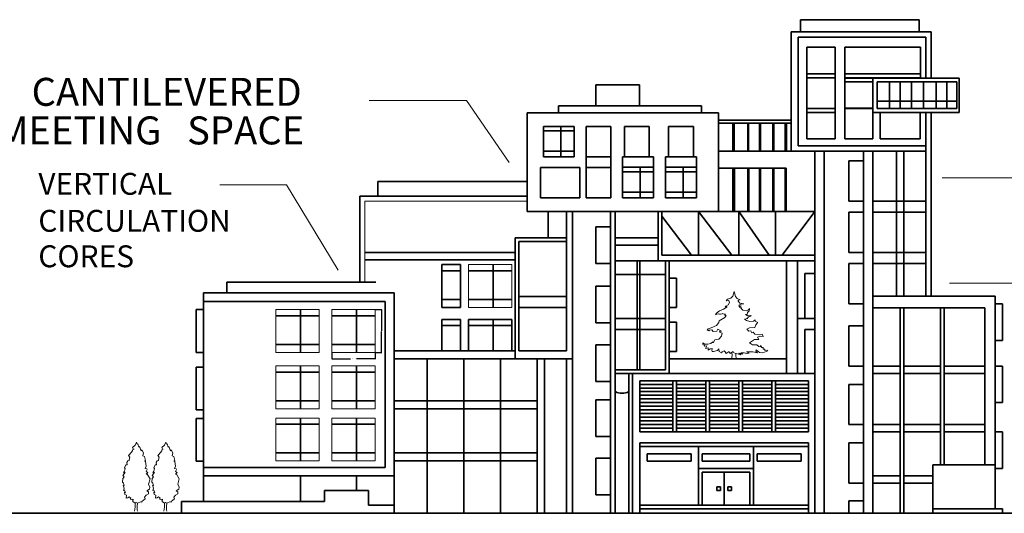
# Model space of a CAD drawing. Units: inches. Extents: x -1080 to 1950, y -1929 to 857.
# Tile 15 of 16: x 769 to 1335, y 9 to 293. Entities that reach past the tile are written whole.
import ezdxf

# ---------------------------------------------------------------- set-up
doc = ezdxf.new("R2010")
doc.units = ezdxf.units.IN
doc.header["$MEASUREMENT"] = 0
for name, color, linetype, lineweight in [('A-ANNO-DIMS', 2, 'Continuous', 18), ('A-ANNO-SYMB', 2, 'Continuous', 18), ('A-ANNO-TEXT', 7, 'Continuous', 25), ('A-ELEV', 7, 'Continuous', 35), ('A-GLAZ', 4, 'Continuous', 18), ('L-PLNT', 82, 'Continuous', 13)]:
    doc.layers.add(name, color=color, linetype=linetype, lineweight=lineweight)
doc.styles.get("Standard").update_dxf_attribs({"font": 'arial.ttf'})
doc.dimstyles.get("Standard").update_dxf_attribs({"dimtxt": 0.18, "dimasz": 0.18, "dimexe": 0.18, "dimexo": 0.0625, "dimgap": 0.09, "dimtad": 0, "dimtih": 1, "dimtoh": 1, "dimdec": 4, "dimzin": 0, "dimdsep": 46, "dimtxsty": 'Standard', "dimcen": 0.09, "dimadec": 0, "dimazin": 0, "dimtfac": 1, "dimtdec": 4, "dimtofl": 0, "dimtmove": 0, "dimatfit": 3, "dimfxl": 1, "dimtolj": 1, "dimtzin": 0, "dimarcsym": 0})

# ---------------------------------------------------------------- blocks, each defined once
blk = doc.blocks.new('*U11')
blk.add_lwpolyline([(-69.9516, 4869.1546), (-172.212, 4644.4154), (-347.5228, 4494.6062), (-303.6824, 4400.9564), (-245.2624, 4382.2366), (-362.1278, 4326.0518), (-347.5228, 4251.1472), (-552.0182, 4007.6882), (-639.6736, 3932.7836), (-537.4132, 3820.414), (-552.0182, 3745.5094), (-581.2536, 3576.955), (-668.8836, 3558.2098), (-741.934, 3427.1204), (-727.329, 3277.3112), (-829.5894, 3258.5914), (-917.2194, 3052.572), (-873.4044, 3015.1324), (-902.6144, 2827.8582), (-990.2698, 2696.7434), (-873.4044, 2734.2084), (-1034.0848, 2509.4692), (-946.4294, 2434.5646), (-1034.0848, 2303.4752), (-1048.6898, 2041.2964), (-975.6648, 1985.1116), (-931.8244, 1797.8374), (-1004.8748, 1816.5572), (-946.4294, 1629.283), (-975.6648, 1460.7286), (-917.2194, 1479.4738), (-844.1944, 1329.6392), (-902.6144, 1348.3844), (-888.0094, 1179.83), (-771.144, 1142.365), (-800.354, 917.6512), (-668.8836, 936.371), (-595.8586, 1011.2756), (-464.3882, 917.6512), (-508.2032, 842.7212), (-376.7328, 805.2816), (-303.6824, 842.7212), (-318.2874, 692.912), (-157.607, 580.5424), (-99.187, 618.0074), (3.0734, 580.5424), (207.5942, 674.1922), (295.2496, 636.7272), (309.8546, 692.912), (543.56, 880.1862), (499.745, 992.5558), (602.0054, 1142.365), (762.6858, 1217.2696), (777.2908, 1367.1042), (645.8204, 1442.0088), (835.7362, 1554.3784), (864.9462, 1704.1876), (777.2908, 1910.207), (879.5512, 2284.7554), (675.0304, 2621.8388), (602.0054, 2621.8388), (718.8708, 2734.2084), (602.0054, 2809.113), (675.0304, 2940.2024), (645.8204, 2996.3872), (528.955, 3015.1324), (616.6104, 3164.9416), (572.7954, 3502.0504), (485.14, 3539.49), (572.7954, 3576.955), (499.745, 3857.8536), (368.2746, 3895.3186), (412.0896, 4120.0578), (309.8546, 4326.0518), (266.0142, 4251.1472), (149.1488, 4550.791), (105.3338, 4513.326), (17.6784, 4756.785), (-11.5316, 4719.32)], close=True)
for points in [[(-173.0502, 601.1926), (-173.0502, 296.3926), (-219.1258, 0)], [(9.8298, 601.1926), (-14.6304, 337.0834), (-14.6304, 93.6244), (0, 0)]]:
    blk.add_lwpolyline(points)
blk = doc.blocks.new('*U7')
blk.add_lwpolyline([(-69.9516, 4869.1546), (-172.212, 4644.4154), (-347.5228, 4494.6062), (-303.6824, 4400.9564), (-245.2624, 4382.2366), (-362.1278, 4326.0518), (-347.5228, 4251.1472), (-552.0182, 4007.6882), (-639.6736, 3932.7836), (-537.4132, 3820.414), (-552.0182, 3745.5094), (-581.2536, 3576.955), (-668.8836, 3558.2098), (-741.934, 3427.1204), (-727.329, 3277.3112), (-829.5894, 3258.5914), (-917.2194, 3052.572), (-873.4044, 3015.1324), (-902.6144, 2827.8582), (-990.2698, 2696.7434), (-873.4044, 2734.2084), (-1034.0848, 2509.4692), (-946.4294, 2434.5646), (-1034.0848, 2303.4752), (-1048.6898, 2041.2964), (-975.6648, 1985.1116), (-931.8244, 1797.8374), (-1004.8748, 1816.5572), (-946.4294, 1629.283), (-975.6648, 1460.7286), (-917.2194, 1479.4738), (-844.1944, 1329.6392), (-902.6144, 1348.3844), (-888.0094, 1179.83), (-771.144, 1142.365), (-800.354, 917.6512), (-668.8836, 936.371), (-595.8586, 1011.2756), (-464.3882, 917.6512), (-508.2032, 842.7212), (-376.7328, 805.2816), (-303.6824, 842.7212), (-318.2874, 692.912), (-157.607, 580.5424), (-99.187, 618.0074), (3.0734, 580.5424), (207.5942, 674.1922), (295.2496, 636.7272), (309.8546, 692.912), (543.56, 880.1862), (499.745, 992.5558), (602.0054, 1142.365), (762.6858, 1217.2696), (777.2908, 1367.1042), (645.8204, 1442.0088), (835.7362, 1554.3784), (864.9462, 1704.1876), (777.2908, 1910.207), (879.5512, 2284.7554), (675.0304, 2621.8388), (602.0054, 2621.8388), (718.8708, 2734.2084), (602.0054, 2809.113), (675.0304, 2940.2024), (645.8204, 2996.3872), (528.955, 3015.1324), (616.6104, 3164.9416), (572.7954, 3502.0504), (485.14, 3539.49), (572.7954, 3576.955), (499.745, 3857.8536), (368.2746, 3895.3186), (412.0896, 4120.0578), (309.8546, 4326.0518), (266.0142, 4251.1472), (149.1488, 4550.791), (105.3338, 4513.326), (17.6784, 4756.785), (-11.5316, 4719.32)], close=True)
for points in [[(-173.0502, 601.1926), (-173.0502, 296.3926), (-219.1258, 0)], [(9.8298, 601.1926), (-14.6304, 337.0834), (-14.6304, 93.6244), (0, 0)]]:
    blk.add_lwpolyline(points)
blk = doc.blocks.new('*U10')
for p, q in [((-247.65, 0), (-209.8802, 192.9892)), ((-209.8802, 192.9892), (-222.1738, 358.267)), ((-19.5834, 242.824), (-17.526, 300.5582)), ((0, 0), (-19.5834, 242.824))]:
    blk.add_line(p, q)
for points in [[(-99.06, 3615.69), (-167.5384, 3353.7398), (-274.3454, 3262.4522), (-452.374, 3201.5938), (-523.5956, 3110.2808), (-452.374, 3140.71), (-381.1778, 3125.4954), (-345.567, 3018.9932), (-428.6504, 2897.251), (-547.3446, 2821.178), (-582.9554, 2790.7488), (-487.9848, 2805.9634), (-499.872, 2775.5342), (-666.0388, 2669.0066), (-879.6782, 2577.719), (-1045.845, 2456.0022), (-1105.1794, 2364.6892), (-1045.845, 2395.1184), (-939.0126, 2425.5476), (-879.6782, 2395.1184), (-832.2056, 2395.1184), (-749.1222, 2425.5476)], [(-95.4786, 3606.038), (-27.2796, 3343.7322), (61.8998, 3229.3814), (224.536, 3162.1222), (166.8272, 3162.1222), (103.886, 3128.4926), (109.1184, 3094.8884), (198.2978, 2993.9996), (408.1526, 2946.908), (266.4968, 2926.7404), (140.589, 2879.6488), (177.3174, 2866.2122), (151.0792, 2819.1206), (261.2644, 2846.0192), (172.085, 2778.7854), (297.9928, 2745.1558), (250.7742, 2724.9628), (350.4438, 2603.9064), (555.0408, 2570.2768), (659.9682, 2637.536), (712.4192, 2704.7952), (707.1868, 2671.1656), (696.6966, 2577.0078), (612.7496, 2482.85), (586.5114, 2375.2302), (497.332, 2375.2302), (597.027, 2328.164), (717.677, 2307.9964), (812.1142, 2334.895), (738.6574, 2281.0724), (623.2398, 2254.1738), (680.9486, 2240.7372), (570.7888, 2186.9146), (633.73, 2173.478), (439.6232, 2139.8484), (555.0408, 2052.4216), (738.6574, 2012.061), (932.7642, 2032.2286), (1011.4534, 2092.7568), (1016.7112, 2032.2286), (1153.1092, 1944.8018)], [(-742.95, 2426.97), (-642.2898, 2395.1184), (-559.2064, 2395.1184), (-606.679, 2319.0454), (-523.5956, 2319.0454), (-594.8172, 2212.5432), (-903.4018, 2045.1572), (-915.289, 1953.8696), (-1045.845, 1786.4836), (-1330.6806, 1664.7668), (-1496.8474, 1619.0976), (-1544.32, 1558.2392), (-1449.3748, 1512.5954), (-1425.6512, 1543.0246), (-1295.0698, 1558.2392), (-1223.8736, 1466.9516), (-1033.9578, 1497.3808), (-974.6234, 1588.6684), (-772.8458, 1482.1662), (-855.9292, 1482.1662), (-891.54, 1436.5224), (-749.1222, 1375.6386), (-784.7076, 1223.4926), (-915.289, 1056.1066), (-1128.9284, 1025.6774), (-1223.8736, 858.2914), (-1247.5972, 919.1752), (-1342.5678, 827.8622), (-1508.7346, 797.433), (-1663.0142, 797.433), (-1781.7084, 873.506), (-1769.8466, 782.2184), (-1698.625, 736.5746), (-1674.9014, 690.9308), (-1556.2072, 706.1454), (-1639.2906, 569.1886), (-1484.9856, 599.6178), (-1484.9856, 477.901), (-1378.1532, 538.7594), (-1259.4844, 553.974), (-1295.0698, 477.901), (-1283.208, 401.828), (-1200.1246, 401.828), (-998.3724, 462.6864), (-927.1508, 538.7594), (-903.4018, 401.828), (-772.8458, 340.9442), (-749.1222, 386.6134), (-642.2898, 432.2572), (-582.9554, 386.6134), (-535.4574, 295.3004), (-369.2906, 401.828), (-333.7052, 295.3004), (-155.6512, 401.828), (-120.0404, 325.7296), (259.7404, 234.442), (141.0716, 310.515), (342.8238, 264.8712), (259.7404, 325.7296), (425.9072, 340.9442), (568.3504, 295.3004), (698.9064, 310.515), (556.4886, 386.6134), (888.8222, 386.6134), (1138.0724, 325.7296), (1054.989, 417.0426), (1078.7126, 493.1156), (1244.8794, 356.1842), (1434.7698, 340.9442), (1695.9072, 432.2572), (1636.5474, 477.901), (1529.7404, 462.6864), (1529.7404, 523.5448), (1446.657, 523.5448), (1446.657, 614.8324), (1375.4354, 614.8324), (1304.2392, 721.36), (1280.4902, 660.5016), (1209.2686, 675.7162), (1114.3234, 767.0038), (983.7674, 767.0038), (876.935, 767.0038), (710.7682, 858.2914), (983.7674, 1040.892), (1209.2686, 1040.892), (1149.9342, 1162.6342), (1327.9628, 1223.4926), (1446.657, 1208.278), (1399.1844, 1329.9948), (1233.0176, 1299.5656), (995.6292, 1329.9948), (912.5458, 1436.5224), (841.3242, 1406.0678), (793.8516, 1512.5954), (687.0446, 1482.1662), (568.3504, 1588.6684), (722.6554, 1664.7668), (995.6292, 1695.196), (1054.989, 1832.1274), (1149.9342, 1938.655)]]:
    blk.add_lwpolyline(points)
blk = doc.blocks.new('WIN-SQUARE')
for p, q in [((0, 24.67), (0, 0)), ((24.91, 24.67), (0, 24.67)), ((24.91, 0), (24.91, 24.67)), ((0, 0), (24.91, 0))]:
    blk.add_line(p, q)
blk = doc.blocks.new('*D69')
at = {"layer": 'A-ANNO-DIMS', "color": 0, "lineweight": -2, "transparency": 16777216}
for p, q in [((948.5, 101.5), (948.5, 97.65)), ((948.68, 97.83), (959.27, 97.83)), ((973.22, 97.83), (962.63, 97.83)), ((973.4, 101.5), (973.4, 97.65))]:
    blk.add_line(p, q, dxfattribs=at)
at = {"layer": 'A-ANNO-DIMS', "color": 0, "transparency": 16777216}
for points in [[(948.68, 97.86), (948.68, 97.8), (948.5, 97.83)], [(973.22, 97.86), (973.22, 97.8), (973.4, 97.83)]]:
    blk.add_solid(points, dxfattribs=at)
at = {"layer": 'Defpoints', "color": 0, "transparency": 16777216}
for p in [(948.5, 101.56), (973.4, 101.56), (973.4, 97.83)]:
    blk.add_point(p, dxfattribs=at)
at = {"layer": 'A-ANNO-DIMS', "color": 0, "transparency": 16777216, "insert": (960.95, 97.83), "char_height": 0.18, "attachment_point": 5}
blk.add_mtext('\\A1;SQUARE WINDOW 25 TYP.', dxfattribs=at)
blk = doc.blocks.new('*D70')
at = {"layer": 'A-ANNO-DIMS', "color": 0, "lineweight": -2, "transparency": 16777216}
for p, q in [((973.47, 126.24), (977.32, 126.24)), ((977.14, 126.06), (977.14, 114.08)), ((977.14, 101.74), (977.14, 113.72)), ((973.47, 101.56), (977.32, 101.56))]:
    blk.add_line(p, q, dxfattribs=at)
at = {"layer": 'A-ANNO-DIMS', "color": 0, "transparency": 16777216}
for points in [[(977.11, 126.06), (977.17, 126.06), (977.14, 126.24)], [(977.11, 101.74), (977.17, 101.74), (977.14, 101.56)]]:
    blk.add_solid(points, dxfattribs=at)
at = {"layer": 'Defpoints', "color": 0, "transparency": 16777216}
for p in [(973.4, 126.24), (977.14, 126.24), (973.4, 101.56)]:
    blk.add_point(p, dxfattribs=at)
at = {"layer": 'A-ANNO-DIMS', "color": 0, "transparency": 16777216, "insert": (977.14, 113.9), "char_height": 0.18, "attachment_point": 5}
blk.add_mtext('\\A1;25 TYP.', dxfattribs=at)

msp = doc.modelspace()

# ---------------------------------------------------------------- linework, layer by layer
at = {"layer": 'A-ANNO-SYMB'}
for p, q in [((1026.06, 246.75), (969.93, 246.75)), ((1050.5, 211.03), (1026.06, 246.75)), ((1299.6, 202.14), (1345.49, 202.14)), ((922.34, 198.18), (884.13, 198.18)), ((952.21, 148.89), (922.34, 198.18)), ((967.5, 142.06), (967.5, 188.65)), ((967.5, 188.65), (1060.92, 188.65)), ((1303.79, 141.55), (1392.21, 141.55))]:
    msp.add_line(p, q, dxfattribs=at)
at = {"layer": 'A-ELEV'}
for p, q in [((1218.17, 286.27), (1218.17, 293.2)), ((1218.17, 293.2), (1286.45, 293.2)), ((1286.45, 293.2), (1286.45, 286.27)), ((1212.83, 217.57), (1212.83, 286.27)), ((1212.83, 286.27), (1293.18, 286.27)), ((1216.68, 283.21), (1290.25, 283.21)), ((1216.68, 220.51), (1216.68, 283.21)), ((1290.25, 283.21), (1290.25, 259.53)), ((1293.18, 286.27), (1293.18, 259.53)), ((1221.83, 277.33), (1238.06, 277.33)), ((1221.83, 224.58), (1221.83, 277.33)), ((1238.06, 277.33), (1238.06, 224.58)), ((1243.54, 277.33), (1243.54, 261.97)), ((1287.05, 277.33), (1243.54, 277.33)), ((1287.05, 261.97), (1287.05, 277.33)), ((1238.06, 261.97), (1221.83, 261.97)), ((1243.54, 261.97), (1287.05, 261.97)), ((1243.54, 261.97), (1243.54, 259.78)), ((1287.05, 259.78), (1287.05, 261.97)), ((1100.35, 243.64), (1100.35, 255.66)), ((1100.35, 255.66), (1120.76, 255.66)), ((1120.76, 255.66), (1125.54, 255.66)), ((1125.54, 255.66), (1125.54, 243.64)), ((1221.83, 259.78), (1238.06, 259.78)), ((1243.54, 259.78), (1287.05, 259.78)), ((1259.79, 259.58), (1243.56, 259.58)), ((1243.56, 242.16), (1243.56, 259.58)), ((1243.56, 257.4), (1259.79, 257.4)), ((1259.79, 242.16), (1259.79, 259.58)), ((1259.79, 259.53), (1309.3, 259.53)), ((1262.15, 242.01), (1262.15, 257.4)), ((1262.15, 257.4), (1308.05, 257.4)), ((1269.3, 242.01), (1269.3, 257.4)), ((1275.49, 242.01), (1275.49, 257.4)), ((1281.96, 242.01), (1281.96, 257.4)), ((1288.77, 242.01), (1288.77, 257.4)), ((1296.22, 242.01), (1296.22, 257.4)), ((1302.24, 242.01), (1302.24, 257.4)), ((1308.05, 257.4), (1308.05, 242.01)), ((1309.3, 259.53), (1309.3, 239.82)), ((1078.84, 239.54), (1078.84, 243.64)), ((1078.84, 243.64), (1161.24, 243.64)), ((1161.24, 243.64), (1161.24, 239.54)), ((1262.15, 246.19), (1308.05, 246.19)), ((1062.14, 239.54), (1060.92, 239.54)), ((1060.92, 239.54), (1060.92, 182.75)), ((1062.14, 239.54), (1170.89, 239.54)), ((1170.89, 182.75), (1170.89, 239.54)), ((1238.06, 242.01), (1221.83, 242.01)), ((1221.83, 239.82), (1238.06, 239.82)), ((1259.79, 242.16), (1243.56, 242.16)), ((1259.79, 242.01), (1243.56, 242.01)), ((1243.56, 224.58), (1243.56, 242.01)), ((1259.79, 224.58), (1259.79, 242.01)), ((1259.79, 239.82), (1280.2, 239.82)), ((1262.15, 239.82), (1261.16, 239.82)), ((1262.15, 242.01), (1308.05, 242.01)), ((1263.97, 224.58), (1263.97, 239.82)), ((1270.77, 239.82), (1287.01, 239.82)), ((1309.3, 239.82), (1287.01, 239.82)), ((1287.01, 224.58), (1287.01, 239.82)), ((1290.25, 239.82), (1290.25, 220.51)), ((1293.18, 239.82), (1293.18, 217.57)), ((1170.89, 235.28), (1212.83, 235.28)), ((1212.83, 233.53), (1170.89, 233.53)), ((1179.2, 233.53), (1179.2, 217.57)), ((1179.95, 233.53), (1179.95, 217.57)), ((1187.73, 233.53), (1187.73, 217.57)), ((1188.29, 233.53), (1188.29, 217.57)), ((1194.49, 233.53), (1194.49, 217.57)), ((1195.07, 233.53), (1195.07, 217.57)), ((1202.18, 233.53), (1202.18, 217.57)), ((1202.77, 233.53), (1202.77, 217.57)), ((1209.32, 233.53), (1209.32, 217.57)), ((1210, 233.53), (1210, 217.57)), ((1070.2, 231.75), (1070.2, 214.15)), ((1087.97, 231.75), (1070.2, 231.75)), ((1070.2, 229.24), (1087.97, 229.24)), ((1080.33, 231.75), (1080.33, 214.15)), ((1087.97, 214.15), (1087.97, 231.75)), ((1094.75, 231.75), (1101.97, 231.75)), ((1094.75, 231.75), (1094.75, 214.15)), ((1109.1, 231.75), (1101.97, 231.75)), ((1109.1, 214.15), (1109.1, 231.75)), ((1116.8, 231.75), (1124.02, 231.75)), ((1116.8, 231.75), (1116.8, 214.15)), ((1131.14, 231.75), (1124.02, 231.75)), ((1131.14, 214.15), (1131.14, 231.75)), ((1142.16, 231.75), (1149.38, 231.75)), ((1142.16, 231.75), (1142.16, 214.15)), ((1156.51, 231.75), (1149.38, 231.75)), ((1156.51, 214.15), (1156.51, 231.75)), ((1238.06, 224.58), (1221.83, 224.58)), ((1243.56, 224.58), (1259.79, 224.58)), ((1280.2, 224.58), (1263.97, 224.58)), ((1287.01, 224.58), (1270.77, 224.58)), ((1070.2, 217.42), (1087.97, 217.42)), ((1170.89, 217.57), (1210, 217.57)), ((1209.32, 217.57), (1212.83, 217.57)), ((1290.25, 217.57), (1209.32, 217.57)), ((1290.25, 220.51), (1216.68, 220.51)), ((1226.29, 195.43), (1226.29, 217.57)), ((1231.69, 217.57), (1231.69, 8.95)), ((1254.27, 217.57), (1254.27, 8.95)), ((1259.79, 217.57), (1259.79, 8.95)), ((1273.24, 134.03), (1273.24, 217.57)), ((1277.46, 134.03), (1277.46, 217.57)), ((1290.25, 220.51), (1290.25, 134.03)), ((1293.18, 217.57), (1293.18, 134.03)), ((1070.2, 214.15), (1087.97, 214.15)), ((1094.75, 214.15), (1109.1, 214.15)), ((1094.75, 208.13), (1094.75, 214.15)), ((1109.1, 208.13), (1109.1, 214.15)), ((1115.81, 208.19), (1115.81, 214.15)), ((1115.81, 214.15), (1115.81, 214.15)), ((1115.81, 214.15), (1116.8, 214.15)), ((1116.8, 214.15), (1131.14, 214.15)), ((1133.58, 214.15), (1131.14, 214.15)), ((1133.58, 208.19), (1133.58, 214.15)), ((1140.49, 208.19), (1140.49, 214.15)), ((1140.49, 214.15), (1141.16, 214.15)), ((1141.16, 214.15), (1155.51, 214.15)), ((1155.51, 214.15), (1158.26, 214.15)), ((1158.26, 214.15), (1158.26, 208.19)), ((1254.27, 211.85), (1245.83, 211.85)), ((1245.83, 211.85), (1245.83, 188.65)), ((1068.53, 208.13), (1068.53, 190.53)), ((1091.11, 208.13), (1068.53, 208.13)), ((1091.11, 190.53), (1091.11, 208.13)), ((1094.75, 208.13), (1101.97, 208.13)), ((1094.75, 208.13), (1094.75, 190.53)), ((1109.1, 208.13), (1101.97, 208.13)), ((1109.1, 190.53), (1109.1, 208.13)), ((1115.81, 208.19), (1115.81, 190.59)), ((1133.58, 208.19), (1115.81, 208.19)), ((1115.81, 205.68), (1133.58, 205.68)), ((1125.94, 208.19), (1125.94, 190.59)), ((1133.58, 190.59), (1133.58, 208.19)), ((1140.49, 208.19), (1140.49, 190.59)), ((1158.26, 208.19), (1140.49, 208.19)), ((1140.49, 205.68), (1158.26, 205.68)), ((1150.62, 208.19), (1150.62, 190.59)), ((1158.26, 190.59), (1158.26, 208.19)), ((1170.89, 207.61), (1209.85, 207.61)), ((1179.2, 207.61), (1179.2, 182.75)), ((1180.08, 207.61), (1180.08, 182.75)), ((1187.73, 207.61), (1187.73, 182.75)), ((1188.44, 207.61), (1188.44, 182.75)), ((1194.49, 207.61), (1194.49, 182.75)), ((1195.07, 207.61), (1195.07, 182.75)), ((1202.18, 207.61), (1202.18, 182.75)), ((1202.7, 207.61), (1202.7, 182.75)), ((1209.32, 207.61), (1209.32, 182.75)), ((1209.85, 207.61), (1209.85, 182.75)), ((974.96, 195.37), (974.96, 199.93)), ((974.96, 199.93), (1060.92, 199.93)), ((974.96, 195.37), (974.96, 191.62)), ((1115.81, 193.86), (1133.58, 193.86)), ((1140.49, 193.86), (1158.26, 193.86)), ((1226.29, 195.43), (1226.29, 193.27)), ((1226.29, 193.27), (1226.29, 8.95)), ((974.96, 191.62), (964.54, 191.62)), ((964.54, 191.62), (964.54, 142.06)), ((974.96, 191.62), (1060.92, 191.62)), ((1091.11, 190.53), (1068.53, 190.53)), ((1094.75, 190.53), (1109.1, 190.53)), ((1115.81, 190.59), (1133.58, 190.59)), ((1140.49, 190.59), (1158.26, 190.59)), ((1245.83, 188.65), (1254.27, 188.65)), ((1259.79, 188.65), (1290.25, 188.65)), ((1060.92, 182.75), (1170.89, 182.75)), ((1072.93, 182.75), (1072.93, 171.78)), ((1083.47, 102.57), (1083.47, 182.75)), ((1086.89, 182.75), (1086.89, 8.95)), ((1108.78, 8.95), (1108.78, 182.75)), ((1111.59, 182.75), (1111.59, 8.95)), ((1136.19, 182.75), (1136.19, 156.4)), ((1138.3, 157.62), (1138.3, 182.75)), ((1159.38, 157.62), (1159.38, 182.75)), ((1159.38, 182.75), (1178.65, 157.62)), ((1170.89, 182.75), (1226.29, 182.75)), ((1182.58, 157.62), (1182.58, 182.75)), ((1182.58, 182.75), (1200.1, 157.62)), ((1203.66, 157.62), (1203.66, 182.75)), ((1226.29, 182.75), (1207.49, 157.62)), ((1254.27, 182.33), (1245.83, 182.33)), ((1245.83, 182.33), (1245.83, 159.13)), ((1259.79, 182.33), (1290.25, 182.33)), ((1138.3, 180), (1155.46, 157.62)), ((1072.93, 171.78), (1072.93, 167.57)), ((1108.78, 173.89), (1100.34, 173.89)), ((1100.34, 173.89), (1100.34, 152.81)), ((1083.47, 167.57), (1053.95, 167.57)), ((1053.95, 167.57), (1053.95, 140.15)), ((1083.47, 165.46), (1056.06, 165.46)), ((1056.06, 165.46), (1056.06, 159.13)), ((1136.19, 167.57), (1111.59, 167.57)), ((1053.95, 159.13), (967.5, 159.13)), ((1056.06, 154.91), (1056.06, 159.13)), ((1136.19, 163.35), (1111.59, 163.35)), ((1245.83, 159.13), (1254.27, 159.13)), ((1259.79, 159.13), (1290.25, 159.13)), ((967.5, 154.91), (1053.95, 154.91)), ((1056.06, 154.91), (1056.06, 102.57)), ((1136.19, 154.29), (1111.59, 154.29)), ((1124.24, 154.29), (1124.24, 146.48)), ((1125.64, 154.29), (1125.64, 146.48)), ((1136.19, 156.4), (1136.19, 154.29)), ((1136.19, 154.29), (1226.29, 154.29)), ((1140.65, 157.62), (1138.3, 157.62)), ((1140.4, 91.66), (1140.4, 154.29)), ((1140.65, 157.62), (1226.29, 157.62)), ((1142.51, 154.29), (1142.51, 89.55)), ((1209.99, 146.48), (1209.99, 154.29)), ((1216.31, 144.37), (1216.31, 154.29)), ((1022.48, 152.18), (1011.78, 152.18)), ((1011.78, 152.18), (1011.78, 127.5)), ((1011.78, 148.66), (1022.48, 148.66)), ((1022.48, 127.5), (1022.48, 152.18)), ((1027.1, 148.66), (1052, 148.66)), ((1041.3, 152.18), (1041.3, 127.5)), ((1100.34, 152.81), (1108.78, 152.81)), ((1254.27, 152.81), (1245.83, 152.81)), ((1245.83, 152.81), (1245.83, 129.61)), ((1259.79, 152.81), (1290.25, 152.81)), ((888.1, 136.6), (888.1, 142.06)), ((888.1, 142.06), (964.54, 142.06)), ((964.54, 142.06), (973.83, 142.06)), ((1140.4, 146.48), (1111.59, 146.48)), ((1124.24, 146.48), (1124.24, 114.85)), ((1125.64, 146.48), (1125.64, 114.85)), ((1142.51, 144.37), (1146.73, 144.37)), ((1146.73, 144.37), (1146.73, 127.5)), ((1209.99, 146.48), (1209.99, 91.66)), ((1216.31, 144.37), (1216.31, 89.55)), ((1220.53, 121.18), (1220.53, 146.95)), ((1220.53, 146.95), (1226.29, 146.95)), ((984.37, 135.94), (874.63, 135.94)), ((874.63, 130.97), (874.63, 135.94)), ((888.1, 136.6), (888.1, 135.94)), ((984.37, 30.51), (984.37, 135.94)), ((1053.95, 140.15), (1053.95, 102.57)), ((1108.78, 139.73), (1100.34, 139.73)), ((1100.34, 139.73), (1100.34, 118.64)), ((888.1, 130.97), (874.63, 130.97)), ((874.63, 130.97), (874.63, 35.3)), ((888.1, 130.97), (979.13, 130.97)), ((979.13, 130.97), (979.13, 35.3)), ((1011.78, 132.09), (1022.48, 132.09)), ((1027.1, 132.09), (1052, 132.09)), ((1083.47, 133.83), (1056.06, 133.83)), ((1259.79, 134.03), (1330.02, 134.03)), ((1290.25, 134.03), (1293.18, 134.03)), ((1293.18, 134.03), (1330.02, 134.03)), ((1330.02, 134.03), (1330.02, 11.53)), ((874.63, 126.24), (870.51, 126.24)), ((870.51, 126.24), (870.51, 101.56)), ((930.45, 126.24), (930.45, 101.56)), ((962.7, 126.24), (962.7, 101.56)), ((1011.78, 127.5), (1022.48, 127.5)), ((1083.47, 127.5), (1056.06, 127.5)), ((1146.73, 127.5), (1142.51, 127.5)), ((1245.83, 129.61), (1254.27, 129.61)), ((1259.79, 127.2), (1322.62, 127.2)), ((1275.35, 8.95), (1275.35, 127.2)), ((1277.46, 127.2), (1277.46, 8.95)), ((1298.55, 36.83), (1298.55, 127.2)), ((1300.66, 127.2), (1300.66, 36.83)), ((1322.62, 127.2), (1324.22, 127.2)), ((1324.22, 127.2), (1324.22, 36.83)), ((1330.02, 129.61), (1334.39, 129.61)), ((1334.39, 129.61), (1334.39, 108.53)), ((916.25, 122.72), (941.15, 122.72)), ((948.5, 122.72), (973.4, 122.72)), ((1022.48, 120.55), (1011.78, 120.55)), ((1011.78, 120.55), (1011.78, 102.57)), ((1022.48, 102.57), (1022.48, 120.55)), ((1027.1, 120.55), (1027.1, 102.57)), ((1052, 120.55), (1027.1, 120.55)), ((1041.3, 120.55), (1041.3, 102.57)), ((1052, 102.57), (1052, 120.55)), ((1140.4, 121.18), (1111.59, 121.18)), ((1142.51, 119.07), (1146.73, 119.07)), ((1146.73, 119.07), (1146.73, 102.2)), ((1216.31, 121.18), (1226.29, 121.18)), ((1011.78, 117.03), (1022.48, 117.03)), ((1027.1, 117.03), (1052, 117.03)), ((1100.34, 118.64), (1108.78, 118.64)), ((1140.4, 114.85), (1111.59, 114.85)), ((1124.24, 114.85), (1124.24, 91.66)), ((1125.64, 114.85), (1125.64, 91.66)), ((1220.53, 89.55), (1220.53, 114.85)), ((1220.53, 114.85), (1226.29, 114.85)), ((1254.27, 116.96), (1245.83, 116.96)), ((1245.83, 116.96), (1245.83, 93.77)), ((1334.39, 108.53), (1330.02, 108.53)), ((916.25, 106.15), (941.15, 106.15)), ((948.5, 106.15), (973.4, 106.15)), ((984.37, 102.57), (1053.95, 102.57)), ((1053.95, 102.57), (1053.95, 97.98)), ((1056.06, 102.57), (1083.47, 102.57)), ((1108.78, 105.99), (1100.34, 105.99)), ((1100.34, 105.99), (1100.34, 84.91)), ((1146.73, 102.2), (1142.51, 102.2)), ((870.51, 101.56), (874.63, 101.56)), ((984.37, 97.98), (1053.95, 97.98)), ((1003.35, 97.98), (1003.35, 8.95)), ((1024.43, 97.98), (1024.43, 8.95)), ((1045.52, 97.98), (1045.52, 8.95)), ((1053.95, 97.98), (1086.89, 97.98)), ((1056.06, 97.98), (1083.47, 97.98)), ((1066.6, 8.95), (1066.6, 97.98)), ((1070.82, 8.95), (1070.82, 97.98)), ((1083.47, 8.95), (1083.47, 97.98)), ((1142.51, 97.98), (1209.99, 97.98)), ((874.63, 93.14), (870.51, 93.14)), ((870.51, 93.14), (870.51, 68.46)), ((930.45, 93.8), (930.45, 69.12)), ((962.7, 93.8), (962.7, 69.12)), ((1111.59, 91.66), (1121.43, 91.66)), ((1121.43, 91.66), (1140.4, 91.66)), ((1209.99, 91.66), (1209.99, 89.55)), ((1245.83, 93.77), (1254.27, 93.77)), ((1259.79, 93.77), (1275.35, 93.77)), ((1277.46, 93.77), (1298.55, 93.77)), ((1300.66, 93.77), (1324.22, 93.77)), ((1330.02, 93.77), (1334.39, 93.77)), ((1334.39, 93.77), (1334.39, 72.68)), ((916.25, 90.28), (941.15, 90.28)), ((948.5, 90.28), (973.4, 90.28)), ((1121.43, 89.55), (1111.59, 89.55)), ((1119.32, 8.95), (1119.32, 89.55)), ((1121.43, 87.44), (1121.43, 89.55)), ((1121.43, 89.55), (1124.24, 89.55)), ((1121.43, 8.95), (1121.43, 87.44)), ((1124.24, 89.55), (1140.4, 89.55)), ((1142.51, 85.33), (1125.64, 85.33)), ((1125.64, 85.33), (1125.64, 55.81)), ((1140.4, 89.55), (1226.29, 89.55)), ((1216.31, 85.33), (1142.51, 85.33)), ((1144.62, 85.33), (1146.73, 85.33)), ((1144.62, 55.81), (1144.62, 85.33)), ((1146.73, 85.33), (1146.73, 55.81)), ((1163.6, 85.33), (1165.71, 85.33)), ((1163.6, 55.81), (1163.6, 85.33)), ((1165.71, 85.33), (1165.71, 55.81)), ((1182.58, 85.33), (1184.68, 85.33)), ((1182.58, 55.81), (1182.58, 85.33)), ((1184.68, 85.33), (1184.68, 55.81)), ((1201.55, 85.33), (1203.66, 85.33)), ((1201.55, 55.81), (1201.55, 85.33)), ((1203.66, 85.33), (1203.66, 55.81)), ((1216.31, 85.33), (1222.64, 85.33)), ((1222.64, 55.81), (1222.64, 85.33)), ((1259.79, 89.55), (1275.35, 89.55)), ((1277.46, 89.55), (1298.55, 89.55)), ((1300.66, 89.55), (1324.22, 89.55)), ((1100.34, 84.91), (1108.78, 84.91)), ((1125.64, 83.22), (1144.62, 83.22)), ((1125.64, 81.11), (1144.62, 81.11)), ((1125.64, 81.11), (1144.62, 81.11)), ((1146.73, 83.22), (1163.6, 83.22)), ((1146.73, 81.11), (1163.6, 81.11)), ((1146.73, 81.11), (1163.6, 81.11)), ((1165.71, 83.22), (1182.58, 83.22)), ((1165.71, 81.11), (1182.58, 81.11)), ((1165.71, 81.11), (1182.58, 81.11)), ((1184.68, 83.22), (1201.55, 83.22)), ((1184.68, 81.11), (1201.55, 81.11)), ((1184.68, 81.11), (1201.55, 81.11)), ((1203.66, 83.22), (1222.64, 83.22)), ((1203.66, 81.11), (1222.64, 81.11)), ((1203.66, 81.11), (1222.64, 81.11)), ((1254.27, 83.22), (1245.83, 83.22)), ((1245.83, 83.22), (1245.83, 60.03)), ((916.25, 73.71), (941.15, 73.71)), ((948.5, 73.71), (973.4, 73.71)), ((984.37, 73.71), (1066.6, 73.71)), ((1108.78, 74.36), (1100.34, 74.36)), ((1100.34, 74.36), (1100.34, 53.28)), ((1125.64, 79.01), (1144.62, 79.01)), ((1125.64, 76.9), (1144.62, 76.9)), ((1125.64, 74.79), (1144.62, 74.79)), ((1146.73, 79.01), (1163.6, 79.01)), ((1146.73, 76.9), (1163.6, 76.9)), ((1146.73, 74.79), (1163.6, 74.79)), ((1165.71, 79.01), (1182.58, 79.01)), ((1165.71, 76.9), (1182.58, 76.9)), ((1165.71, 74.79), (1182.58, 74.79)), ((1184.68, 79.01), (1201.55, 79.01)), ((1184.68, 76.9), (1201.55, 76.9)), ((1184.68, 74.79), (1201.55, 74.79)), ((1203.66, 79.01), (1222.64, 79.01)), ((1203.66, 76.9), (1222.64, 76.9)), ((1203.66, 74.79), (1222.64, 74.79)), ((870.51, 68.46), (874.63, 68.46)), ((984.37, 69.12), (1066.6, 69.12)), ((1125.64, 72.68), (1144.62, 72.68)), ((1125.64, 70.57), (1144.62, 70.57)), ((1125.64, 70.57), (1144.62, 70.57)), ((1125.64, 68.46), (1144.62, 68.46)), ((1146.73, 72.68), (1163.6, 72.68)), ((1146.73, 70.57), (1163.6, 70.57)), ((1146.73, 70.57), (1163.6, 70.57)), ((1146.73, 68.46), (1163.6, 68.46)), ((1165.71, 72.68), (1182.58, 72.68)), ((1165.71, 70.57), (1182.58, 70.57)), ((1165.71, 70.57), (1182.58, 70.57)), ((1165.71, 68.46), (1182.58, 68.46)), ((1184.68, 72.68), (1201.55, 72.68)), ((1184.68, 70.57), (1201.55, 70.57)), ((1184.68, 70.57), (1201.55, 70.57)), ((1184.68, 68.46), (1201.55, 68.46)), ((1203.66, 72.68), (1222.64, 72.68)), ((1203.66, 70.57), (1222.64, 70.57)), ((1203.66, 70.57), (1222.64, 70.57)), ((1203.66, 68.46), (1222.64, 68.46)), ((1334.39, 72.68), (1330.02, 72.68)), ((874.63, 63.62), (870.51, 63.62)), ((870.51, 63.62), (870.51, 38.94)), ((930.45, 63.82), (930.45, 39.14)), ((962.7, 63.82), (962.7, 39.14)), ((1125.64, 66.35), (1144.62, 66.35)), ((1125.64, 64.25), (1144.62, 64.25)), ((1146.73, 66.35), (1163.6, 66.35)), ((1146.73, 64.25), (1163.6, 64.25)), ((1165.71, 66.35), (1182.58, 66.35)), ((1165.71, 64.25), (1182.58, 64.25)), ((1184.68, 66.35), (1201.55, 66.35)), ((1184.68, 64.25), (1201.55, 64.25)), ((1203.66, 66.35), (1222.64, 66.35)), ((1203.66, 64.25), (1222.64, 64.25)), ((916.25, 60.3), (941.15, 60.3)), ((948.5, 60.3), (973.4, 60.3)), ((1125.64, 62.14), (1144.62, 62.14)), ((1125.64, 60.03), (1144.62, 60.03)), ((1125.64, 57.92), (1144.62, 57.92)), ((1146.73, 62.14), (1163.6, 62.14)), ((1146.73, 60.03), (1163.6, 60.03)), ((1146.73, 57.92), (1163.6, 57.92)), ((1165.71, 62.14), (1182.58, 62.14)), ((1165.71, 60.03), (1182.58, 60.03)), ((1165.71, 57.92), (1182.58, 57.92)), ((1184.68, 62.14), (1201.55, 62.14)), ((1184.68, 60.03), (1201.55, 60.03)), ((1184.68, 57.92), (1201.55, 57.92)), ((1203.66, 62.14), (1222.64, 62.14)), ((1203.66, 60.03), (1222.64, 60.03)), ((1203.66, 57.92), (1222.64, 57.92)), ((1245.83, 60.03), (1254.27, 60.03)), ((1259.79, 60.03), (1275.35, 60.03)), ((1277.46, 60.03), (1298.55, 60.03)), ((1300.66, 60.03), (1324.22, 60.03)), ((1100.34, 53.28), (1108.78, 53.28)), ((1125.64, 55.81), (1144.62, 55.81)), ((1144.62, 55.81), (1163.6, 55.81)), ((1163.6, 55.81), (1182.58, 55.81)), ((1182.58, 55.81), (1201.55, 55.81)), ((1201.55, 55.81), (1222.64, 55.81)), ((1259.79, 55.81), (1275.35, 55.81)), ((1277.46, 55.81), (1298.55, 55.81)), ((1300.66, 55.81), (1324.22, 55.81)), ((1330.02, 55.81), (1334.39, 55.81)), ((1334.39, 55.81), (1334.39, 34.73)), ((1125.64, 49.49), (1125.64, 8.95)), ((1125.64, 49.49), (1222.64, 49.49)), ((1125.64, 47.38), (1222.64, 47.38)), ((1159.38, 47.38), (1159.38, 13.64)), ((1191.01, 47.38), (1191.01, 13.64)), ((1222.64, 49.49), (1222.64, 8.95)), ((1254.27, 49.49), (1245.83, 49.49)), ((1245.83, 49.49), (1245.83, 26.29)), ((916.25, 43.73), (941.15, 43.73)), ((948.5, 43.73), (973.4, 43.73)), ((984.37, 43.73), (1066.6, 43.73)), ((1108.78, 40.63), (1100.34, 40.63)), ((1100.34, 40.63), (1100.34, 19.54)), ((1129.86, 43.16), (1129.86, 38.94)), ((1155.16, 43.16), (1129.86, 43.16)), ((1155.16, 38.94), (1155.16, 43.16)), ((1163.6, 43.16), (1161.49, 43.16)), ((1161.49, 43.16), (1161.49, 38.94)), ((1188.9, 43.16), (1163.6, 43.16)), ((1188.9, 38.94), (1188.9, 43.16)), ((1193.12, 43.16), (1193.12, 38.94)), ((1218.42, 43.16), (1193.12, 43.16)), ((1218.42, 38.94), (1218.42, 43.16)), ((870.51, 38.94), (874.63, 38.94)), ((874.63, 35.3), (979.13, 35.3)), ((874.63, 35.3), (874.63, 15.75)), ((984.37, 39.14), (1066.6, 39.14)), ((1129.86, 38.94), (1155.16, 38.94)), ((1159.38, 34.73), (1191.01, 34.73)), ((1161.49, 38.94), (1163.6, 38.94)), ((1163.6, 38.94), (1188.9, 38.94)), ((1193.12, 38.94), (1218.42, 38.94)), ((1294.33, 8.95), (1294.33, 36.83)), ((1294.33, 36.83), (1324.22, 36.83)), ((1324.22, 36.83), (1330.02, 36.83)), ((1334.39, 34.73), (1330.02, 34.73)), ((874.63, 30.51), (984.37, 30.51)), ((930.45, 30.51), (930.45, 15.75)), ((962.7, 30.51), (962.7, 22.07)), ((984.37, 30.51), (984.37, 8.95)), ((1125.64, 30.51), (1125.64, 11.53)), ((1161.49, 32.62), (1161.49, 13.64)), ((1161.49, 32.62), (1188.9, 32.62)), ((1174.14, 13.64), (1174.14, 32.62)), ((1188.9, 32.62), (1188.9, 13.64)), ((1259.79, 30.51), (1275.35, 30.51)), ((1277.46, 30.51), (1294.33, 30.51)), ((1169.92, 24.18), (1169.92, 22.07)), ((1172.03, 24.18), (1169.92, 24.18)), ((1172.03, 22.07), (1172.03, 24.18)), ((1176.25, 24.18), (1176.25, 22.07)), ((1178.36, 24.18), (1176.25, 24.18)), ((1178.36, 22.07), (1178.36, 24.18)), ((1245.83, 26.29), (1254.27, 26.29)), ((1259.79, 26.29), (1275.35, 26.29)), ((1277.46, 26.29), (1294.33, 26.29)), ((944.31, 15.75), (944.31, 22.07)), ((944.31, 22.07), (969.61, 22.07)), ((969.61, 22.07), (969.61, 13.64)), ((1100.34, 19.54), (1108.78, 19.54)), ((1169.92, 22.07), (1172.03, 22.07)), ((1176.25, 22.07), (1178.36, 22.07)), ((862.07, 8.95), (862.07, 15.75)), ((862.07, 15.75), (944.31, 15.75)), ((969.61, 13.64), (984.37, 13.64)), ((1125.64, 13.64), (1222.64, 13.64)), ((1125.64, 11.53), (1222.64, 11.53)), ((1254.27, 16.22), (1245.83, 16.22)), ((1245.83, 16.22), (1245.83, 8.95)), ((1294.33, 11.53), (1334.39, 11.53)), ((1334.39, 11.53), (1334.39, 8.95)), ((709.45, 9.02), (833.43, 9.02)), ((887.28, 8.95), (798.82, 8.95)), ((887.28, 8.95), (1380.78, 8.95)), ((1125.64, 8.95), (1224.75, 8.95)), ((1259.79, 8.95), (1324.22, 8.95)), ((1294.33, 8.95), (1294.33, 8.95))]:
    msp.add_line(p, q, dxfattribs=at)
msp.add_arc((1115.46, 86.5), 8.43, 242.7444, 297.2556, dxfattribs=at)

# ---------------------------------------------------------------- block references
at = {"layer": 'A-GLAZ'}
for p in [(1027.1, 127.5), (916.25, 101.56), (948.5, 101.56), (916.25, 69.12), (948.5, 69.12), (916.25, 39.14), (948.5, 39.14)]:
    msp.add_blockref('WIN-SQUARE', p, dxfattribs=at)
at = {"layer": 'L-PLNT'}
for name, p, xscale, yscale, zscale in [('*U10', (1181.07, 97.78), 0.010774584635974, 0.010774584635974, 0.010774584635974), ('*U7', (836.72, 10.13), 0.0081804086702915, 0.0081804086702915, 0.0081804086702915), ('*U11', (853.59, 10.13), 0.0081804086702915, 0.0081804086702915, 0.0081804086702915)]:
    msp.add_blockref(name, p, dxfattribs=dict(at, xscale=xscale, yscale=yscale, zscale=zscale))

# ---------------------------------------------------------------- texts
at = {"layer": 'A-ANNO-TEXT'}
for s, height, p in [('CANTILEVERED  ', 16.1087, (775.81, 243.59)), ('MEETING   SPACE', 16.1087, (756.13, 221.37)), ('VERTICAL', 12.614, (779.67, 192.37)), ('CIRCULATION', 12.614, (779.67, 171.07)), ('CORES', 12.614, (779.67, 150.64))]:
    msp.add_text(s, height=height, dxfattribs=at).set_placement(p)

# ---------------------------------------------------------------- dimensions: what is measured, and where the dimension line sits
at = {"layer": 'A-ANNO-DIMS'}
dim = msp.add_linear_dim(base=(977.14, 126.24), p1=(973.4, 101.56), p2=(973.4, 126.24), angle=90, text='<> TYP.', dimstyle='Standard', override={"dimdec": 0, "dimlfac": 1, "dimrnd": 0, "dimzin": 0, "dimdsep": 46, "dimlunit": 2}, dxfattribs=at)
dim.commit()
dim.dimension.update_dxf_attribs({"geometry": '*D70', "text_midpoint": (977.14, 113.9)})
dim = msp.add_linear_dim(base=(973.4, 97.83), p1=(948.5, 101.56), p2=(973.4, 101.56), text='SQUARE WINDOW <> TYP.', dimstyle='Standard', override={"dimdec": 0, "dimlfac": 1, "dimrnd": 0, "dimzin": 0, "dimdsep": 46, "dimlunit": 2}, dxfattribs=at)
dim.commit()
dim.dimension.update_dxf_attribs({"geometry": '*D69', "text_midpoint": (960.95, 97.83)})

doc.saveas('drawing.dxf')
